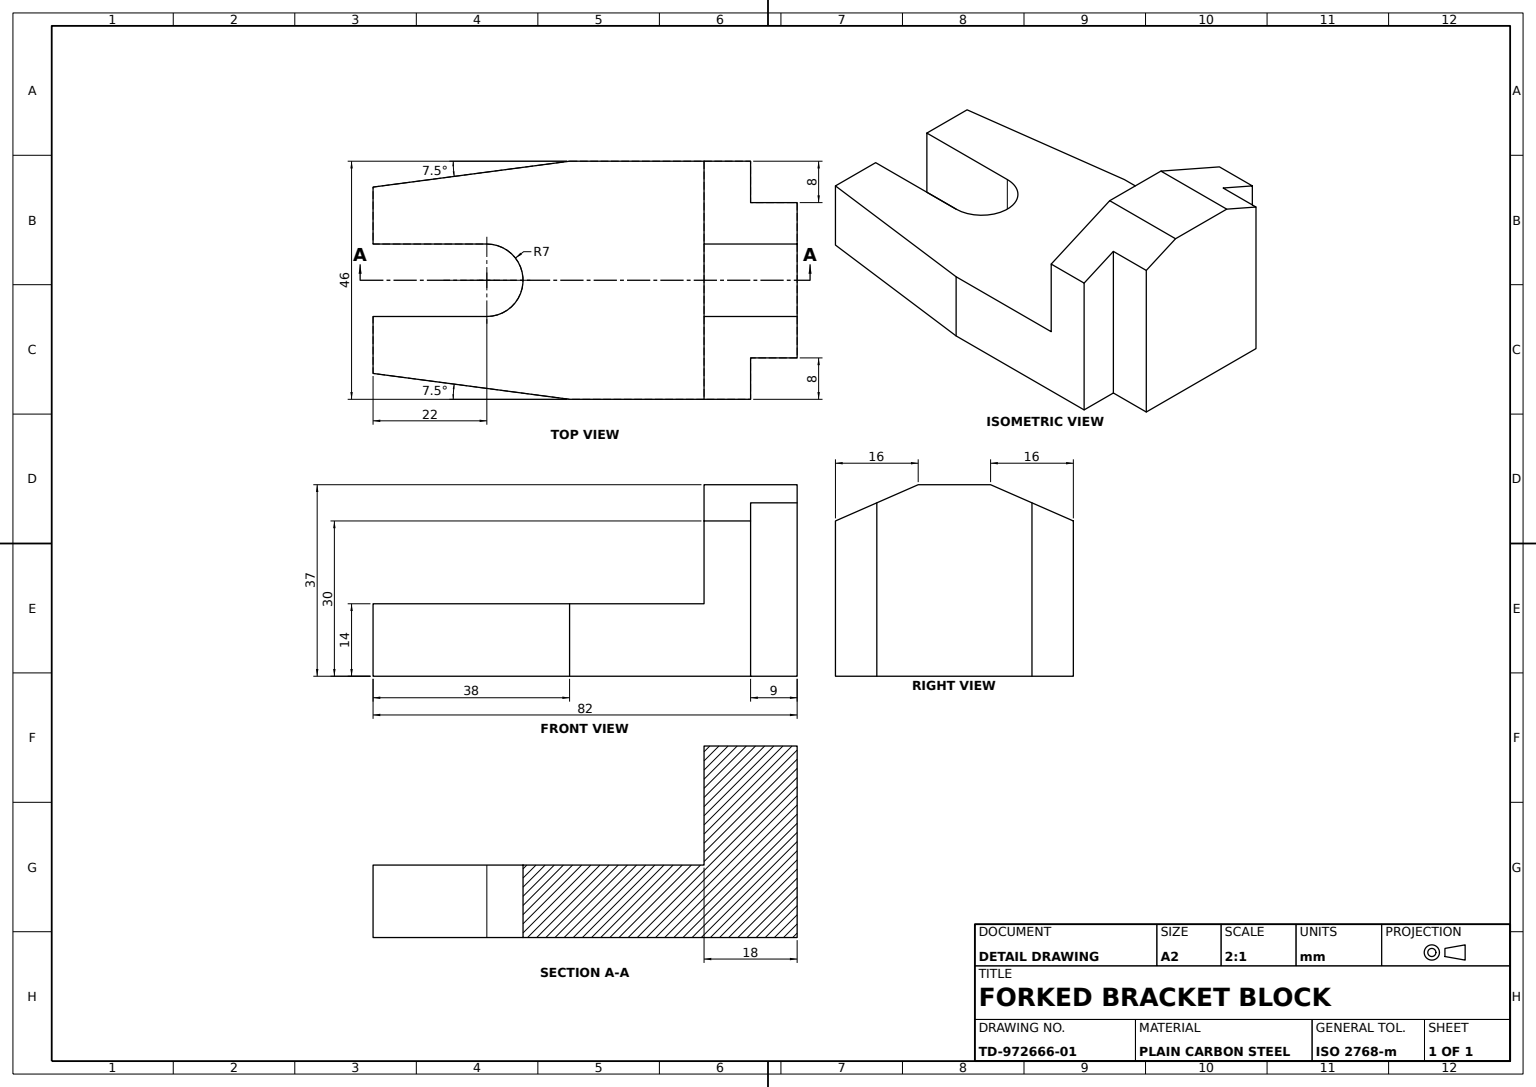
from build123d import *

# Parameters (mm, degrees)
FORKED_BASE_DEPTH   = 18
UPRIGHT_BOSS_DEPTH  = 14
NOTCH_SKETCH_8X9_W  = 8
NOTCH_SKETCH_8X9_H  = 9
NOTCH_CUT_8X9_DEPTH = 93.854725243


with BuildPart() as part:
    # Base Profile Sketch → Forked Base (new body)
    with BuildSketch(Plane.XY):
        Polygon((-23, 15), (-7, 22), (7, 22), (23, 15), (23, -15), (-23, -15), align=None)
    extrude(amount=FORKED_BASE_DEPTH)

    # Upright Profile Sketch → Upright Boss (add)
    with BuildSketch(Plane(origin=(0, -15, 0), x_dir=(-1, 0, 0), z_dir=(0, -1, 0))):
        with BuildLine():
            Line((-23, -18), (-23, -44))
            Line((-23, -44), (-18, -82))
            Line((-18, -82), (-7, -82))
            Line((-7, -82), (-7, -60))
            ThreePointArc((-7, -60), (0, -53), (7, -60))
            Line((7, -60), (7, -82))
            Line((7, -82), (18, -82))
            Line((18, -82), (23, -44))
            Line((23, -44), (23, -18))
            Line((23, -18), (-23, -18))
        make_face()
    extrude(amount=-UPRIGHT_BOSS_DEPTH)

    # Notch Sketch 8x9 → Notch Cut 8x9 (cut, through all)
    with BuildSketch(Plane.XZ.offset(15)):
        with Locations((19, 4.5)):
            Rectangle(NOTCH_SKETCH_8X9_W, NOTCH_SKETCH_8X9_H)
    notch_cut_8x9 = extrude(amount=-NOTCH_CUT_8X9_DEPTH, mode=Mode.SUBTRACT)

    # Notch Mirror: Notch Cut 8x9 across plane
    add(notch_cut_8x9.mirror(Plane(origin=(0, 0, 0), x_dir=(0, 0, 1), z_dir=(1, 0, 0))), mode=Mode.SUBTRACT)


solid = part.part
